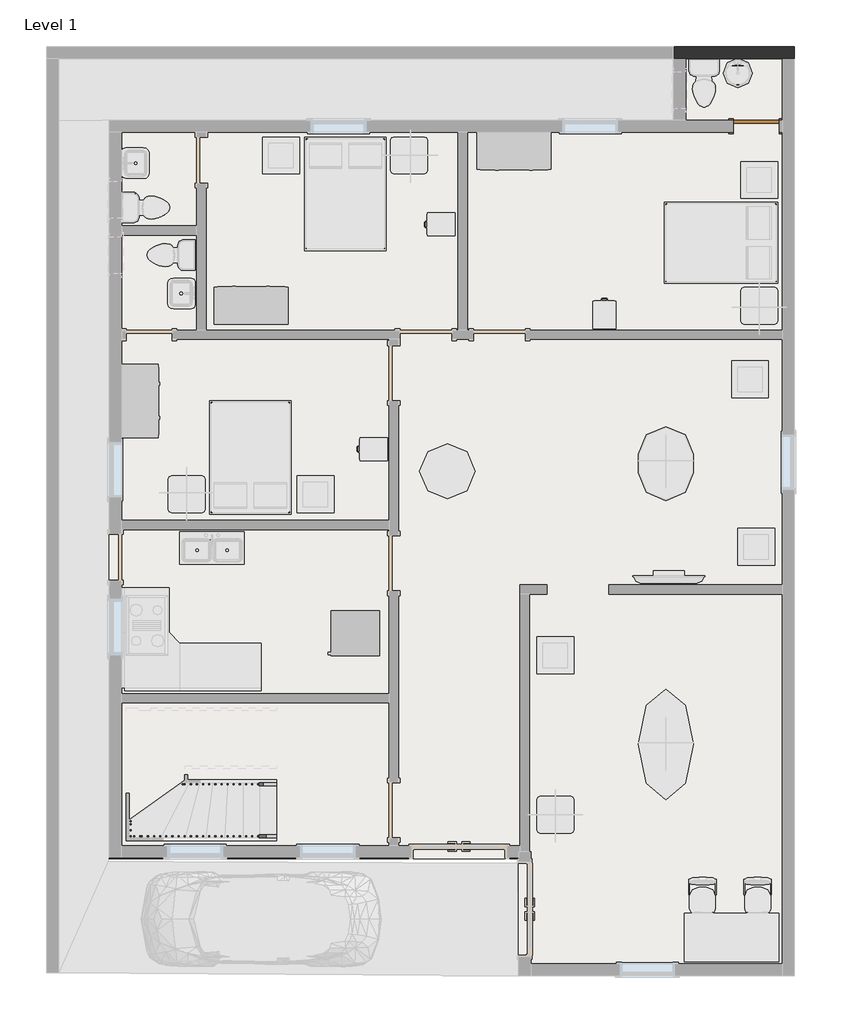
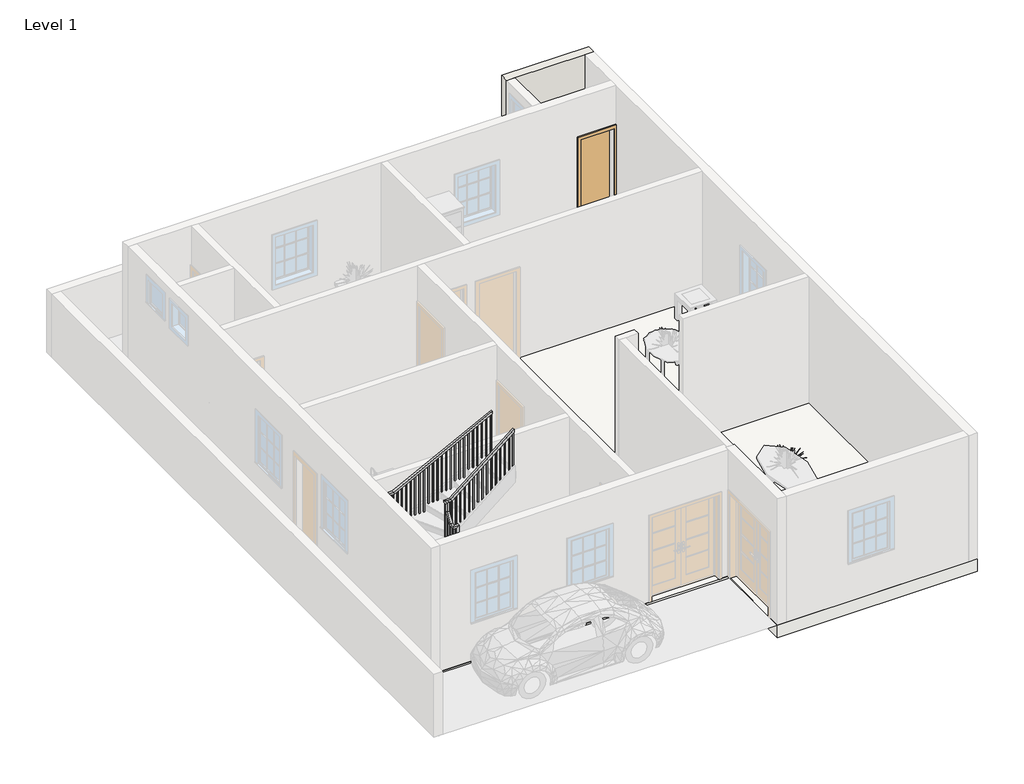
# One storey, part 2 of 3: 2 railings, 2 slabs, 1 door, 1 wall.
"""IFC4 building model written with IfcOpenShell, lengths in millimetres."""

from ifc_helpers import new_model, si_unit, frame, origin, place, context, project, spatial, polyline, outline, extrude, faceted_brep, transform, mapped, element, save
from components import door_fadea3f2

model = new_model("IFC4")

# Units and contexts
model_context = context("Model", 3, world=origin())
ifc_project = project(units=[si_unit("LENGTHUNIT", "METRE", prefix="MILLI")], contexts=[model_context])

# Site, building, storey
site = spatial("IfcSite", under=ifc_project)
building = spatial("IfcBuilding", under=site)
storey = spatial("IfcBuildingStorey", under=building, Name="Level 1", Elevation=0.0)

# Door
placement = place(None, origin())
door_shape = door_fadea3f2(model_context)
element("IfcDoor", 1, ObjectType="Single-Flush : 30\" x 80\"", at=placement, inside=storey, context=model_context, shape_type="MappedRepresentation", body=[
    mapped(door_shape, transform((2172.6442798, 14156.4245992, 0.0), x_axis=(1.0, 0.0, 0.0), y_axis=(0.0, 1.0, 0.0), z_axis=(0.0, 0.0, 1.0))),
])

# Railings
element("IfcRailing", 2, ObjectType="Handrail - Rectangular", at=placement, inside=storey, context=model_context, shape_type="SolidModel", body=[
    faceted_brep([(-5773.8240284, 3234.4245992, 1025.2529681), (-5773.8240284, 3234.4245992, 959.7067088), (-5773.8240284, 3285.2245992, 959.7067088), (-5773.8240284, 3285.2245992, 1025.2529681), (-7225.3557202, 3234.4245992, 2208.7848338), (-7276.1557202, 3234.4245992, 2184.659247), (-7276.1557202, 3285.2245992, 2184.659247), (-7225.3557202, 3285.2245992, 2208.7848338), (-7225.3557202, 3234.4245992, 2414.6281882), (-7276.1557202, 3234.4245992, 2363.8281882), (-7276.1557202, 3285.2245992, 2363.8281882), (-7225.3557202, 3285.2245992, 2414.6281882), (-7352.3557202, 3234.4245992, 2414.6281882), (-7352.3557202, 3234.4245992, 2363.8281882), (-7301.5557202, 3285.2245992, 2363.8281882), (-7301.5557202, 3285.2245992, 2414.6281882), (-7352.3557202, 3361.4245992, 2414.6281882), (-7352.3557202, 3390.5459331, 2363.8281882), (-7301.5557202, 3390.5459331, 2363.8281882), (-7301.5557202, 3361.4245992, 2414.6281882), (-7352.3557202, 3488.4245992, 2631.5051451), (-7352.3557202, 3539.2245992, 2617.7256424), (-7301.5557202, 3539.2245992, 2617.7256424), (-7301.5557202, 3488.4245992, 2631.5051451), (-7352.3557202, 3488.4245992, 2837.3484995), (-7352.3557202, 3539.2245992, 2786.5484995), (-7301.5557202, 3539.2245992, 2786.5484995), (-7301.5557202, 3488.4245992, 2837.3484995), (-7352.3557202, 3615.4245992, 2837.3484995), (-7352.3557202, 3615.4245992, 2786.5484995), (-7301.5557202, 3564.6245992, 2786.5484995), (-7301.5557202, 3564.6245992, 2837.3484995), (-7225.3557202, 3615.4245992, 2837.3484995), (-7207.2703071, 3615.4245992, 2786.5484995), (-7207.2703071, 3564.6245992, 2786.5484995), (-7225.3557202, 3564.6245992, 2837.3484995), (-5773.8240284, 3615.4245992, 4020.8803652), (-5773.8240284, 3564.6245992, 4020.8803652), (-5773.8240284, 3564.6245992, 3955.3341059), (-5773.8240284, 3615.4245992, 3955.3341059)], [[[0, 1, 2, 3]], [[1, 0, 4, 5]], [[2, 1, 5, 6]], [[3, 2, 6, 7]], [[0, 3, 7, 4]], [[5, 4, 8, 9]], [[6, 5, 9, 10]], [[7, 6, 10, 11]], [[4, 7, 11, 8]], [[9, 8, 12, 13]], [[10, 9, 13, 14]], [[11, 10, 14, 15]], [[8, 11, 15, 12]], [[13, 12, 16, 17]], [[14, 13, 17, 18]], [[15, 14, 18, 19]], [[12, 15, 19, 16]], [[17, 16, 20, 21]], [[18, 17, 21, 22]], [[19, 18, 22, 23]], [[16, 19, 23, 20]], [[21, 20, 24, 25]], [[22, 21, 25, 26]], [[23, 22, 26, 27]], [[20, 23, 27, 24]], [[25, 24, 28, 29]], [[26, 25, 29, 30]], [[27, 26, 30, 31]], [[24, 27, 31, 28]], [[29, 28, 32, 33]], [[30, 29, 33, 34]], [[31, 30, 34, 35]], [[28, 31, 35, 32]], [[36, 37, 38, 39]], [[33, 32, 36, 39]], [[34, 33, 39, 38]], [[35, 34, 38, 37]], [[32, 35, 37, 36]]]),
    extrude(outline(polyline([(3881.7558784, -5864.0633639), (3866.2231262, -5883.1133639), (2878.6666667, -5883.1133639), (2878.6666667, -5864.0633639), (3881.7558784, -5864.0633639)])), frame((0.0, 3580.4995992, 0.0), z_axis=(0.0, 1.0, 0.0), x_axis=(0.0, 0.0, 1.0)), (0.0, 0.0, 1.0), 19.05),
    extrude(outline(polyline([(3798.9145334, -5965.6633639), (3783.3817813, -5984.7133639), (2878.6666667, -5984.7133639), (2878.6666667, -5965.6633639), (3798.9145334, -5965.6633639)])), frame((0.0, 3580.4995992, 0.0), z_axis=(0.0, 1.0, 0.0), x_axis=(0.0, 0.0, 1.0)), (0.0, 0.0, 1.0), 19.05),
    extrude(outline(polyline([(3716.0731885, -6067.2633639), (3700.5404364, -6086.3133639), (2709.3333333, -6086.3133639), (2709.3333333, -6067.2633639), (3716.0731885, -6067.2633639)])), frame((0.0, 3580.4995992, 0.0), z_axis=(0.0, 1.0, 0.0), x_axis=(0.0, 0.0, 1.0)), (0.0, 0.0, 1.0), 19.05),
    extrude(outline(polyline([(3633.2318436, -6168.8633639), (3617.6990914, -6187.9133639), (2709.3333333, -6187.9133639), (2709.3333333, -6168.8633639), (3633.2318436, -6168.8633639)])), frame((0.0, 3580.4995992, 0.0), z_axis=(0.0, 1.0, 0.0), x_axis=(0.0, 0.0, 1.0)), (0.0, 0.0, 1.0), 19.05),
    extrude(outline(polyline([(3550.3904987, -6270.4633639), (3534.8577465, -6289.5133639), (2709.3333333, -6289.5133639), (2709.3333333, -6270.4633639), (3550.3904987, -6270.4633639)])), frame((0.0, 3580.4995992, 0.0), z_axis=(0.0, 1.0, 0.0), x_axis=(0.0, 0.0, 1.0)), (0.0, 0.0, 1.0), 19.05),
    extrude(outline(polyline([(3467.5491538, -6372.0633639), (3452.0164016, -6391.1133639), (2540.0, -6391.1133639), (2540.0, -6372.0633639), (3467.5491538, -6372.0633639)])), frame((0.0, 3580.4995992, 0.0), z_axis=(0.0, 1.0, 0.0), x_axis=(0.0, 0.0, 1.0)), (0.0, 0.0, 1.0), 19.05),
    extrude(outline(polyline([(3384.7078088, -6473.6633639), (3369.1750567, -6492.7133639), (2540.0, -6492.7133639), (2540.0, -6473.6633639), (3384.7078088, -6473.6633639)])), frame((0.0, 3580.4995992, 0.0), z_axis=(0.0, 1.0, 0.0), x_axis=(0.0, 0.0, 1.0)), (0.0, 0.0, 1.0), 19.05),
    extrude(outline(polyline([(3301.8664639, -6575.2633639), (3286.3337117, -6594.3133639), (2540.0, -6594.3133639), (2540.0, -6575.2633639), (3301.8664639, -6575.2633639)])), frame((0.0, 3580.4995992, 0.0), z_axis=(0.0, 1.0, 0.0), x_axis=(0.0, 0.0, 1.0)), (0.0, 0.0, 1.0), 19.05),
    extrude(outline(polyline([(3219.025119, -6676.8633639), (3203.4923668, -6695.9133639), (2370.6666667, -6695.9133639), (2370.6666667, -6676.8633639), (3219.025119, -6676.8633639)])), frame((0.0, 3580.4995992, 0.0), z_axis=(0.0, 1.0, 0.0), x_axis=(0.0, 0.0, 1.0)), (0.0, 0.0, 1.0), 19.05),
    extrude(outline(polyline([(3136.1837741, -6778.4633639), (3120.6510219, -6797.5133639), (2370.6666667, -6797.5133639), (2370.6666667, -6778.4633639), (3136.1837741, -6778.4633639)])), frame((0.0, 3580.4995992, 0.0), z_axis=(0.0, 1.0, 0.0), x_axis=(0.0, 0.0, 1.0)), (0.0, 0.0, 1.0), 19.05),
    extrude(outline(polyline([(3053.3424291, -6880.0633639), (3037.809677, -6899.1133639), (2201.3333333, -6899.1133639), (2201.3333333, -6880.0633639), (3053.3424291, -6880.0633639)])), frame((0.0, 3580.4995992, 0.0), z_axis=(0.0, 1.0, 0.0), x_axis=(0.0, 0.0, 1.0)), (0.0, 0.0, 1.0), 19.05),
    extrude(outline(polyline([(2970.5010842, -6981.6633639), (2954.9683321, -7000.7133639), (2201.3333333, -7000.7133639), (2201.3333333, -6981.6633639), (2970.5010842, -6981.6633639)])), frame((0.0, 3580.4995992, 0.0), z_axis=(0.0, 1.0, 0.0), x_axis=(0.0, 0.0, 1.0)), (0.0, 0.0, 1.0), 19.05),
    extrude(outline(polyline([(2887.6597393, -7083.2633639), (2872.1269871, -7102.3133639), (2032.0, -7102.3133639), (2032.0, -7083.2633639), (2887.6597393, -7083.2633639)])), frame((0.0, 3580.4995992, 0.0), z_axis=(0.0, 1.0, 0.0), x_axis=(0.0, 0.0, 1.0)), (0.0, 0.0, 1.0), 19.05),
    extrude(outline(polyline([(2804.8183944, -7184.8633639), (2789.2856422, -7203.9133639), (2032.0, -7203.9133639), (2032.0, -7184.8633639), (2804.8183944, -7184.8633639)])), frame((0.0, 3580.4995992, 0.0), z_axis=(0.0, 1.0, 0.0), x_axis=(0.0, 0.0, 1.0)), (0.0, 0.0, 1.0), 19.05),
    extrude(outline(polyline([(3468.285503, 2496.5834745), (3487.335503, 2529.115018), (3487.335503, 1524.0), (3468.285503, 1524.0), (3468.285503, 2496.5834745)])), frame((-7336.4807202, 0.0, 0.0), z_axis=(1.0, 0.0, 0.0), x_axis=(0.0, 1.0, 0.0)), (0.0, 0.0, 1.0), 19.05),
    extrude(outline(polyline([(3366.685503, 2323.0819089), (3385.735503, 2355.6134525), (3385.735503, 1524.0), (3366.685503, 1524.0), (3366.685503, 2323.0819089)])), frame((-7336.4807202, 0.0, 0.0), z_axis=(1.0, 0.0, 0.0), x_axis=(0.0, 1.0, 0.0)), (0.0, 0.0, 1.0), 19.05),
    extrude(outline(polyline([(2111.7191617, -7186.6990284), (2127.2519138, -7205.7490284), (1016.0, -7205.7490284), (1016.0, -7186.6990284), (2111.7191617, -7186.6990284)])), frame((0.0, 3250.2995992, 0.0), z_axis=(0.0, 1.0, 0.0), x_axis=(0.0, 0.0, 1.0)), (0.0, 0.0, 1.0), 19.05),
    extrude(outline(polyline([(2028.8778167, -7085.0990284), (2044.4105689, -7104.1490284), (1016.0, -7104.1490284), (1016.0, -7085.0990284), (2028.8778167, -7085.0990284)])), frame((0.0, 3250.2995992, 0.0), z_axis=(0.0, 1.0, 0.0), x_axis=(0.0, 0.0, 1.0)), (0.0, 0.0, 1.0), 19.05),
    extrude(outline(polyline([(1946.0364718, -6983.4990284), (1961.569224, -7002.5490284), (846.6666667, -7002.5490284), (846.6666667, -6983.4990284), (1946.0364718, -6983.4990284)])), frame((0.0, 3250.2995992, 0.0), z_axis=(0.0, 1.0, 0.0), x_axis=(0.0, 0.0, 1.0)), (0.0, 0.0, 1.0), 19.05),
    extrude(outline(polyline([(1863.1951269, -6881.8990284), (1878.7278791, -6900.9490284), (846.6666667, -6900.9490284), (846.6666667, -6881.8990284), (1863.1951269, -6881.8990284)])), frame((0.0, 3250.2995992, 0.0), z_axis=(0.0, 1.0, 0.0), x_axis=(0.0, 0.0, 1.0)), (0.0, 0.0, 1.0), 19.05),
    extrude(outline(polyline([(1780.353782, -6780.2990284), (1795.8865341, -6799.3490284), (677.3333333, -6799.3490284), (677.3333333, -6780.2990284), (1780.353782, -6780.2990284)])), frame((0.0, 3250.2995992, 0.0), z_axis=(0.0, 1.0, 0.0), x_axis=(0.0, 0.0, 1.0)), (0.0, 0.0, 1.0), 19.05),
    extrude(outline(polyline([(1697.5124371, -6678.6990284), (1713.0451892, -6697.7490284), (677.3333333, -6697.7490284), (677.3333333, -6678.6990284), (1697.5124371, -6678.6990284)])), frame((0.0, 3250.2995992, 0.0), z_axis=(0.0, 1.0, 0.0), x_axis=(0.0, 0.0, 1.0)), (0.0, 0.0, 1.0), 19.05),
    extrude(outline(polyline([(1614.6710921, -6577.0990284), (1630.2038443, -6596.1490284), (508.0, -6596.1490284), (508.0, -6577.0990284), (1614.6710921, -6577.0990284)])), frame((0.0, 3250.2995992, 0.0), z_axis=(0.0, 1.0, 0.0), x_axis=(0.0, 0.0, 1.0)), (0.0, 0.0, 1.0), 19.05),
    extrude(outline(polyline([(1531.8297472, -6475.4990284), (1547.3624994, -6494.5490284), (508.0, -6494.5490284), (508.0, -6475.4990284), (1531.8297472, -6475.4990284)])), frame((0.0, 3250.2995992, 0.0), z_axis=(0.0, 1.0, 0.0), x_axis=(0.0, 0.0, 1.0)), (0.0, 0.0, 1.0), 19.05),
    extrude(outline(polyline([(1448.9884023, -6373.8990284), (1464.5211545, -6392.9490284), (508.0, -6392.9490284), (508.0, -6373.8990284), (1448.9884023, -6373.8990284)])), frame((0.0, 3250.2995992, 0.0), z_axis=(0.0, 1.0, 0.0), x_axis=(0.0, 0.0, 1.0)), (0.0, 0.0, 1.0), 19.05),
    extrude(outline(polyline([(1366.1470574, -6272.2990284), (1381.6798095, -6291.3490284), (338.6666667, -6291.3490284), (338.6666667, -6272.2990284), (1366.1470574, -6272.2990284)])), frame((0.0, 3250.2995992, 0.0), z_axis=(0.0, 1.0, 0.0), x_axis=(0.0, 0.0, 1.0)), (0.0, 0.0, 1.0), 19.05),
    extrude(outline(polyline([(1283.3057124, -6170.6990284), (1298.8384646, -6189.7490284), (338.6666667, -6189.7490284), (338.6666667, -6170.6990284), (1283.3057124, -6170.6990284)])), frame((0.0, 3250.2995992, 0.0), z_axis=(0.0, 1.0, 0.0), x_axis=(0.0, 0.0, 1.0)), (0.0, 0.0, 1.0), 19.05),
    extrude(outline(polyline([(1200.4643675, -6069.0990284), (1215.9971197, -6088.1490284), (338.6666667, -6088.1490284), (338.6666667, -6069.0990284), (1200.4643675, -6069.0990284)])), frame((0.0, 3250.2995992, 0.0), z_axis=(0.0, 1.0, 0.0), x_axis=(0.0, 0.0, 1.0)), (0.0, 0.0, 1.0), 19.05),
    extrude(outline(polyline([(1117.6230226, -5967.4990284), (1133.1557748, -5986.5490284), (169.3333333, -5986.5490284), (169.3333333, -5967.4990284), (1117.6230226, -5967.4990284)])), frame((0.0, 3250.2995992, 0.0), z_axis=(0.0, 1.0, 0.0), x_axis=(0.0, 0.0, 1.0)), (0.0, 0.0, 1.0), 19.05),
    extrude(outline(polyline([(1034.7816777, -5865.8990284), (1050.3144298, -5884.9490284), (169.3333333, -5884.9490284), (169.3333333, -5865.8990284), (1034.7816777, -5865.8990284)])), frame((0.0, 3250.2995992, 0.0), z_axis=(0.0, 1.0, 0.0), x_axis=(0.0, 0.0, 1.0)), (0.0, 0.0, 1.0), 19.05),
    extrude(outline(polyline([(-7305.5133639, 3580.4995992), (-7305.5133639, 3599.5495992), (-7286.4633639, 3599.5495992), (-7286.4633639, 3580.4995992), (-7305.5133639, 3580.4995992)])), frame((0.0, 0.0, 1862.6666667), z_axis=(0.0, 0.0, 1.0), x_axis=(1.0, 0.0, 0.0)), (0.0, 0.0, 1.0), 923.8818329),
    extrude(outline(polyline([(-7317.4307202, 3580.4995992), (-7336.4807202, 3580.4995992), (-7336.4807202, 3599.5495992), (-7317.4307202, 3599.5495992), (-7317.4307202, 3580.4995992)])), frame((0.0, 0.0, 1862.6666667), z_axis=(0.0, 0.0, 1.0), x_axis=(1.0, 0.0, 0.0)), (0.0, 0.0, 1.0), 923.8818329),
    extrude(outline(polyline([(-7317.4307202, 3565.7136955), (-7336.4807202, 3565.7136955), (-7336.4807202, 3584.7636955), (-7317.4307202, 3584.7636955), (-7317.4307202, 3565.7136955)])), frame((0.0, 0.0, 1693.3333333), z_axis=(0.0, 0.0, 1.0), x_axis=(1.0, 0.0, 0.0)), (0.0, 0.0, 1.0), 1093.2151662),
    extrude(outline(polyline([(-7317.4307202, 3265.085503), (-7336.4807202, 3265.085503), (-7336.4807202, 3284.135503), (-7317.4307202, 3284.135503), (-7317.4307202, 3265.085503)])), frame((0.0, 0.0, 1354.6666667), z_axis=(0.0, 0.0, 1.0), x_axis=(1.0, 0.0, 0.0)), (0.0, 0.0, 1.0), 1009.1615215),
    extrude(outline(polyline([(-7317.4307202, 3269.3495992), (-7317.4307202, 3250.2995992), (-7336.4807202, 3250.2995992), (-7336.4807202, 3269.3495992), (-7317.4307202, 3269.3495992)])), frame((0.0, 0.0, 1185.3333333), z_axis=(0.0, 0.0, 1.0), x_axis=(1.0, 0.0, 0.0)), (0.0, 0.0, 1.0), 1178.4948549),
    extrude(outline(polyline([(-7286.4633639, 3269.3495992), (-7286.4633639, 3250.2995992), (-7305.5133639, 3250.2995992), (-7305.5133639, 3269.3495992), (-7286.4633639, 3269.3495992)])), frame((0.0, 0.0, 1185.3333333), z_axis=(0.0, 0.0, 1.0), x_axis=(1.0, 0.0, 0.0)), (0.0, 0.0, 1.0), 1178.4948549),
    extrude(outline(polyline([(3955.3341059, -5773.8240284), (3939.8013537, -5792.8740284), (2878.6666667, -5792.8740284), (2878.6666667, -5773.8240284), (3955.3341059, -5773.8240284)])), frame((0.0, 3580.4995992, 0.0), z_axis=(0.0, 1.0, 0.0), x_axis=(0.0, 0.0, 1.0)), (0.0, 0.0, 1.0), 19.05),
    extrude(outline(polyline([(959.7067088, -5773.8240284), (975.239461, -5792.8740284), (169.3333333, -5792.8740284), (169.3333333, -5773.8240284), (959.7067088, -5773.8240284)])), frame((0.0, 3250.2995992, 0.0), z_axis=(0.0, 1.0, 0.0), x_axis=(0.0, 0.0, 1.0)), (0.0, 0.0, 1.0), 19.05),
])
element("IfcRailing", 3, ObjectType="Handrail - Rectangular", at=placement, inside=storey, context=model_context, shape_type="SolidModel", body=[
    faceted_brep([(-5773.8240284, 2370.8245992, 1109.0771751), (-5773.8240284, 2370.8245992, 1051.9280057), (-5773.8240284, 2421.6245992, 1051.9280057), (-5773.8240284, 2421.6245992, 1109.0771751), (-8033.8058849, 2370.8245992, 2273.7644996), (-8046.1259362, 2370.8245992, 2222.9644996), (-8046.1259362, 2421.6245992, 2222.9644996), (-8033.8058849, 2421.6245992, 2273.7644996), (-8215.9557202, 2370.8245992, 2273.7644996), (-8215.9557202, 2370.8245992, 2222.9644996), (-8165.1557202, 2421.6245992, 2222.9644996), (-8165.1557202, 2421.6245992, 2273.7644996), (-8215.9557202, 2647.9785518, 2273.7644996), (-8215.9557202, 2655.929128, 2222.9644996), (-8165.1557202, 2655.929128, 2222.9644996), (-8165.1557202, 2647.9785518, 2273.7644996), (-8215.9557202, 4201.8706466, 2772.3688337), (-8215.9557202, 4209.8212227, 2721.5688337), (-8165.1557202, 4209.8212227, 2721.5688337), (-8165.1557202, 4201.8706466, 2772.3688337), (-8215.9557202, 4479.0245992, 2772.3688337), (-8215.9557202, 4479.0245992, 2721.5688337), (-8165.1557202, 4428.2245992, 2721.5688337), (-8165.1557202, 4428.2245992, 2772.3688337), (-8033.8058849, 4479.0245992, 2772.3688337), (-8021.4858336, 4479.0245992, 2721.5688337), (-8021.4858336, 4428.2245992, 2721.5688337), (-8033.8058849, 4428.2245992, 2772.3688337), (-5773.8240284, 4479.0245992, 3937.0561582), (-5773.8240284, 4428.2245992, 3937.0561582), (-5773.8240284, 4428.2245992, 3879.9069889), (-5773.8240284, 4479.0245992, 3879.9069889)], [[[0, 1, 2, 3]], [[1, 0, 4, 5]], [[2, 1, 5, 6]], [[3, 2, 6, 7]], [[0, 3, 7, 4]], [[5, 4, 8, 9]], [[6, 5, 9, 10]], [[7, 6, 10, 11]], [[4, 7, 11, 8]], [[9, 8, 12, 13]], [[10, 9, 13, 14]], [[11, 10, 14, 15]], [[8, 11, 15, 12]], [[13, 12, 16, 17]], [[14, 13, 17, 18]], [[15, 14, 18, 19]], [[12, 15, 19, 16]], [[17, 16, 20, 21]], [[18, 17, 21, 22]], [[19, 18, 22, 23]], [[16, 19, 23, 20]], [[21, 20, 24, 25]], [[22, 21, 25, 26]], [[23, 22, 26, 27]], [[20, 23, 27, 24]], [[28, 29, 30, 31]], [[25, 24, 28, 31]], [[26, 25, 31, 30]], [[27, 26, 30, 29]], [[24, 27, 29, 28]]]),
    extrude(outline(polyline([(3862.2268642, -5808.1308849), (2878.6666667, -5808.1308849), (2878.6666667, -5789.0808849), (3872.0443296, -5789.0808849), (3862.2268642, -5808.1308849)])), frame((0.0, 4444.0995992, 0.0), z_axis=(0.0, 1.0, 0.0), x_axis=(0.0, 0.0, 1.0)), (0.0, 0.0, 1.0), 19.05),
    extrude(outline(polyline([(3809.8670491, -5909.7308849), (2878.6666667, -5909.7308849), (2878.6666667, -5890.6808849), (3819.6845145, -5890.6808849), (3809.8670491, -5909.7308849)])), frame((0.0, 4444.0995992, 0.0), z_axis=(0.0, 1.0, 0.0), x_axis=(0.0, 0.0, 1.0)), (0.0, 0.0, 1.0), 19.05),
    extrude(outline(polyline([(3757.507234, -6011.3308849), (2878.6666667, -6011.3308849), (2878.6666667, -5992.2808849), (3767.3246993, -5992.2808849), (3757.507234, -6011.3308849)])), frame((0.0, 4444.0995992, 0.0), z_axis=(0.0, 1.0, 0.0), x_axis=(0.0, 0.0, 1.0)), (0.0, 0.0, 1.0), 19.05),
    extrude(outline(polyline([(3705.1474189, -6112.9308849), (2709.3333333, -6112.9308849), (2709.3333333, -6093.8808849), (3714.9648842, -6093.8808849), (3705.1474189, -6112.9308849)])), frame((0.0, 4444.0995992, 0.0), z_axis=(0.0, 1.0, 0.0), x_axis=(0.0, 0.0, 1.0)), (0.0, 0.0, 1.0), 19.05),
    extrude(outline(polyline([(3652.7876038, -6214.5308849), (2709.3333333, -6214.5308849), (2709.3333333, -6195.4808849), (3662.6050691, -6195.4808849), (3652.7876038, -6214.5308849)])), frame((0.0, 4444.0995992, 0.0), z_axis=(0.0, 1.0, 0.0), x_axis=(0.0, 0.0, 1.0)), (0.0, 0.0, 1.0), 19.05),
    extrude(outline(polyline([(3600.4277887, -6316.1308849), (2709.3333333, -6316.1308849), (2709.3333333, -6297.0808849), (3610.245254, -6297.0808849), (3600.4277887, -6316.1308849)])), frame((0.0, 4444.0995992, 0.0), z_axis=(0.0, 1.0, 0.0), x_axis=(0.0, 0.0, 1.0)), (0.0, 0.0, 1.0), 19.05),
    extrude(outline(polyline([(3548.0679735, -6417.7308849), (2540.0, -6417.7308849), (2540.0, -6398.6808849), (3557.8854389, -6398.6808849), (3548.0679735, -6417.7308849)])), frame((0.0, 4444.0995992, 0.0), z_axis=(0.0, 1.0, 0.0), x_axis=(0.0, 0.0, 1.0)), (0.0, 0.0, 1.0), 19.05),
    extrude(outline(polyline([(3495.7081584, -6519.3308849), (2540.0, -6519.3308849), (2540.0, -6500.2808849), (3505.5256238, -6500.2808849), (3495.7081584, -6519.3308849)])), frame((0.0, 4444.0995992, 0.0), z_axis=(0.0, 1.0, 0.0), x_axis=(0.0, 0.0, 1.0)), (0.0, 0.0, 1.0), 19.05),
    extrude(outline(polyline([(3443.3483433, -6620.9308849), (2540.0, -6620.9308849), (2540.0, -6601.8808849), (3453.1658086, -6601.8808849), (3443.3483433, -6620.9308849)])), frame((0.0, 4444.0995992, 0.0), z_axis=(0.0, 1.0, 0.0), x_axis=(0.0, 0.0, 1.0)), (0.0, 0.0, 1.0), 19.05),
    extrude(outline(polyline([(3390.9885282, -6722.5308849), (2370.6666667, -6722.5308849), (2370.6666667, -6703.4808849), (3400.8059935, -6703.4808849), (3390.9885282, -6722.5308849)])), frame((0.0, 4444.0995992, 0.0), z_axis=(0.0, 1.0, 0.0), x_axis=(0.0, 0.0, 1.0)), (0.0, 0.0, 1.0), 19.05),
    extrude(outline(polyline([(3338.6287131, -6824.1308849), (2370.6666667, -6824.1308849), (2370.6666667, -6805.0808849), (3348.4461784, -6805.0808849), (3338.6287131, -6824.1308849)])), frame((0.0, 4444.0995992, 0.0), z_axis=(0.0, 1.0, 0.0), x_axis=(0.0, 0.0, 1.0)), (0.0, 0.0, 1.0), 19.05),
    extrude(outline(polyline([(3286.268898, -6925.7308849), (2370.6666667, -6925.7308849), (2370.6666667, -6906.6808849), (3296.0863633, -6906.6808849), (3286.268898, -6925.7308849)])), frame((0.0, 4444.0995992, 0.0), z_axis=(0.0, 1.0, 0.0), x_axis=(0.0, 0.0, 1.0)), (0.0, 0.0, 1.0), 19.05),
    extrude(outline(polyline([(3233.9090828, -7027.3308849), (2201.3333333, -7027.3308849), (2201.3333333, -7008.2808849), (3243.7265482, -7008.2808849), (3233.9090828, -7027.3308849)])), frame((0.0, 4444.0995992, 0.0), z_axis=(0.0, 1.0, 0.0), x_axis=(0.0, 0.0, 1.0)), (0.0, 0.0, 1.0), 19.05),
    extrude(outline(polyline([(3181.5492677, -7128.9308849), (2201.3333333, -7128.9308849), (2201.3333333, -7109.8808849), (3191.3667331, -7109.8808849), (3181.5492677, -7128.9308849)])), frame((0.0, 4444.0995992, 0.0), z_axis=(0.0, 1.0, 0.0), x_axis=(0.0, 0.0, 1.0)), (0.0, 0.0, 1.0), 19.05),
    extrude(outline(polyline([(3129.1894526, -7230.5308849), (2201.3333333, -7230.5308849), (2201.3333333, -7211.4808849), (3139.0069179, -7211.4808849), (3129.1894526, -7230.5308849)])), frame((0.0, 4444.0995992, 0.0), z_axis=(0.0, 1.0, 0.0), x_axis=(0.0, 0.0, 1.0)), (0.0, 0.0, 1.0), 19.05),
    extrude(outline(polyline([(3076.8296375, -7332.1308849), (2032.0, -7332.1308849), (2032.0, -7313.0808849), (3086.6471028, -7313.0808849), (3076.8296375, -7332.1308849)])), frame((0.0, 4444.0995992, 0.0), z_axis=(0.0, 1.0, 0.0), x_axis=(0.0, 0.0, 1.0)), (0.0, 0.0, 1.0), 19.05),
    extrude(outline(polyline([(3024.4698224, -7433.7308849), (2032.0, -7433.7308849), (2032.0, -7414.6808849), (3034.2872877, -7414.6808849), (3024.4698224, -7433.7308849)])), frame((0.0, 4444.0995992, 0.0), z_axis=(0.0, 1.0, 0.0), x_axis=(0.0, 0.0, 1.0)), (0.0, 0.0, 1.0), 19.05),
    extrude(outline(polyline([(2972.1100073, -7535.3308849), (2032.0, -7535.3308849), (2032.0, -7516.2808849), (2981.9274726, -7516.2808849), (2972.1100073, -7535.3308849)])), frame((0.0, 4444.0995992, 0.0), z_axis=(0.0, 1.0, 0.0), x_axis=(0.0, 0.0, 1.0)), (0.0, 0.0, 1.0), 19.05),
    extrude(outline(polyline([(2919.7501921, -7636.9308849), (2032.0, -7636.9308849), (2032.0, -7617.8808849), (2929.5676575, -7617.8808849), (2919.7501921, -7636.9308849)])), frame((0.0, 4444.0995992, 0.0), z_axis=(0.0, 1.0, 0.0), x_axis=(0.0, 0.0, 1.0)), (0.0, 0.0, 1.0), 19.05),
    extrude(outline(polyline([(2867.390377, -7738.5308849), (1862.6666667, -7738.5308849), (1862.6666667, -7719.4808849), (2877.2078424, -7719.4808849), (2867.390377, -7738.5308849)])), frame((0.0, 4444.0995992, 0.0), z_axis=(0.0, 1.0, 0.0), x_axis=(0.0, 0.0, 1.0)), (0.0, 0.0, 1.0), 19.05),
    extrude(outline(polyline([(2815.0305619, -7840.1308849), (1862.6666667, -7840.1308849), (1862.6666667, -7821.0808849), (2824.8480272, -7821.0808849), (2815.0305619, -7840.1308849)])), frame((0.0, 4444.0995992, 0.0), z_axis=(0.0, 1.0, 0.0), x_axis=(0.0, 0.0, 1.0)), (0.0, 0.0, 1.0), 19.05),
    extrude(outline(polyline([(2762.6707468, -7941.7308849), (1862.6666667, -7941.7308849), (1862.6666667, -7922.6808849), (2772.4882121, -7922.6808849), (2762.6707468, -7941.7308849)])), frame((0.0, 4444.0995992, 0.0), z_axis=(0.0, 1.0, 0.0), x_axis=(0.0, 0.0, 1.0)), (0.0, 0.0, 1.0), 19.05),
    extrude(outline(polyline([(-8098.4807202, 4463.1495992), (-8079.4307202, 4463.1495992), (-8079.4307202, 4444.0995992), (-8098.4807202, 4444.0995992), (-8098.4807202, 4463.1495992)])), frame((0.0, 0.0, 1862.6666667), z_axis=(0.0, 0.0, 1.0), x_axis=(1.0, 0.0, 0.0)), (0.0, 0.0, 1.0), 858.902167),
    extrude(outline(polyline([(-8200.0807202, 4395.5456466), (-8200.0807202, 4414.5956466), (-8181.0307202, 4414.5956466), (-8181.0307202, 4395.5456466), (-8200.0807202, 4395.5456466)])), frame((0.0, 0.0, 1862.6666667), z_axis=(0.0, 0.0, 1.0), x_axis=(1.0, 0.0, 0.0)), (0.0, 0.0, 1.0), 858.902167),
    extrude(outline(polyline([(-8200.0807202, 4293.9456466), (-8200.0807202, 4312.9956466), (-8181.0307202, 4312.9956466), (-8181.0307202, 4293.9456466), (-8200.0807202, 4293.9456466)])), frame((0.0, 0.0, 1862.6666667), z_axis=(0.0, 0.0, 1.0), x_axis=(1.0, 0.0, 0.0)), (0.0, 0.0, 1.0), 858.902167),
    extrude(outline(polyline([(4181.5035518, 2712.4824155), (4181.5035518, 1693.3333333), (4162.4535518, 1693.3333333), (4162.4535518, 2706.3697564), (4181.5035518, 2712.4824155)])), frame((-8200.0807202, 0.0, 0.0), z_axis=(1.0, 0.0, 0.0), x_axis=(0.0, 1.0, 0.0)), (0.0, 0.0, 1.0), 19.05),
    extrude(outline(polyline([(4079.9035518, 2679.8815673), (4079.9035518, 1693.3333333), (4060.8535518, 1693.3333333), (4060.8535518, 2673.7689082), (4079.9035518, 2679.8815673)])), frame((-8200.0807202, 0.0, 0.0), z_axis=(1.0, 0.0, 0.0), x_axis=(0.0, 1.0, 0.0)), (0.0, 0.0, 1.0), 19.05),
    extrude(outline(polyline([(3978.3035518, 2647.280719), (3978.3035518, 1693.3333333), (3959.2535518, 1693.3333333), (3959.2535518, 2641.16806), (3978.3035518, 2647.280719)])), frame((-8200.0807202, 0.0, 0.0), z_axis=(1.0, 0.0, 0.0), x_axis=(0.0, 1.0, 0.0)), (0.0, 0.0, 1.0), 19.05),
    extrude(outline(polyline([(3876.7035518, 2614.6798708), (3876.7035518, 1693.3333333), (3857.6535518, 1693.3333333), (3857.6535518, 2608.5672118), (3876.7035518, 2614.6798708)])), frame((-8200.0807202, 0.0, 0.0), z_axis=(1.0, 0.0, 0.0), x_axis=(0.0, 1.0, 0.0)), (0.0, 0.0, 1.0), 19.05),
    extrude(outline(polyline([(3775.1035518, 2582.0790226), (3775.1035518, 1693.3333333), (3756.0535518, 1693.3333333), (3756.0535518, 2575.9663635), (3775.1035518, 2582.0790226)])), frame((-8200.0807202, 0.0, 0.0), z_axis=(1.0, 0.0, 0.0), x_axis=(0.0, 1.0, 0.0)), (0.0, 0.0, 1.0), 19.05),
    extrude(outline(polyline([(3673.5035518, 2549.4781744), (3673.5035518, 1693.3333333), (3654.4535518, 1693.3333333), (3654.4535518, 2543.3655153), (3673.5035518, 2549.4781744)])), frame((-8200.0807202, 0.0, 0.0), z_axis=(1.0, 0.0, 0.0), x_axis=(0.0, 1.0, 0.0)), (0.0, 0.0, 1.0), 19.05),
    extrude(outline(polyline([(3571.9035518, 2516.8773261), (3571.9035518, 1524.0), (3552.8535518, 1524.0), (3552.8535518, 2510.7646671), (3571.9035518, 2516.8773261)])), frame((-8200.0807202, 0.0, 0.0), z_axis=(1.0, 0.0, 0.0), x_axis=(0.0, 1.0, 0.0)), (0.0, 0.0, 1.0), 19.05),
    extrude(outline(polyline([(3470.3035518, 2484.2764779), (3470.3035518, 1524.0), (3451.2535518, 1524.0), (3451.2535518, 2478.1638189), (3470.3035518, 2484.2764779)])), frame((-8200.0807202, 0.0, 0.0), z_axis=(1.0, 0.0, 0.0), x_axis=(0.0, 1.0, 0.0)), (0.0, 0.0, 1.0), 19.05),
    extrude(outline(polyline([(3368.7035518, 2451.6756297), (3368.7035518, 1524.0), (3349.6535518, 1524.0), (3349.6535518, 2445.5629706), (3368.7035518, 2451.6756297)])), frame((-8200.0807202, 0.0, 0.0), z_axis=(1.0, 0.0, 0.0), x_axis=(0.0, 1.0, 0.0)), (0.0, 0.0, 1.0), 19.05),
    extrude(outline(polyline([(3267.1035518, 2419.0747814), (3267.1035518, 1524.0), (3248.0535518, 1524.0), (3248.0535518, 2412.9621224), (3267.1035518, 2419.0747814)])), frame((-8200.0807202, 0.0, 0.0), z_axis=(1.0, 0.0, 0.0), x_axis=(0.0, 1.0, 0.0)), (0.0, 0.0, 1.0), 19.05),
    extrude(outline(polyline([(3165.5035518, 2386.4739332), (3165.5035518, 1354.6666667), (3146.4535518, 1354.6666667), (3146.4535518, 2380.3612742), (3165.5035518, 2386.4739332)])), frame((-8200.0807202, 0.0, 0.0), z_axis=(1.0, 0.0, 0.0), x_axis=(0.0, 1.0, 0.0)), (0.0, 0.0, 1.0), 19.05),
    extrude(outline(polyline([(3063.9035518, 2353.873085), (3063.9035518, 1354.6666667), (3044.8535518, 1354.6666667), (3044.8535518, 2347.7604259), (3063.9035518, 2353.873085)])), frame((-8200.0807202, 0.0, 0.0), z_axis=(1.0, 0.0, 0.0), x_axis=(0.0, 1.0, 0.0)), (0.0, 0.0, 1.0), 19.05),
    extrude(outline(polyline([(2962.3035518, 2321.2722368), (2962.3035518, 1354.6666667), (2943.2535518, 1354.6666667), (2943.2535518, 2315.1595777), (2962.3035518, 2321.2722368)])), frame((-8200.0807202, 0.0, 0.0), z_axis=(1.0, 0.0, 0.0), x_axis=(0.0, 1.0, 0.0)), (0.0, 0.0, 1.0), 19.05),
    extrude(outline(polyline([(2860.7035518, 2288.6713885), (2860.7035518, 1354.6666667), (2841.6535518, 1354.6666667), (2841.6535518, 2282.5587295), (2860.7035518, 2288.6713885)])), frame((-8200.0807202, 0.0, 0.0), z_axis=(1.0, 0.0, 0.0), x_axis=(0.0, 1.0, 0.0)), (0.0, 0.0, 1.0), 19.05),
    extrude(outline(polyline([(2759.1035518, 2256.0705403), (2759.1035518, 1354.6666667), (2740.0535518, 1354.6666667), (2740.0535518, 2249.9578813), (2759.1035518, 2256.0705403)])), frame((-8200.0807202, 0.0, 0.0), z_axis=(1.0, 0.0, 0.0), x_axis=(0.0, 1.0, 0.0)), (0.0, 0.0, 1.0), 19.05),
    extrude(outline(polyline([(-8200.0807202, 2589.8995992), (-8200.0807202, 2608.9495992), (-8181.0307202, 2608.9495992), (-8181.0307202, 2589.8995992), (-8200.0807202, 2589.8995992)])), frame((0.0, 0.0, 1185.3333333), z_axis=(0.0, 0.0, 1.0), x_axis=(1.0, 0.0, 0.0)), (0.0, 0.0, 1.0), 1037.6311663),
    extrude(outline(polyline([(-8200.0807202, 2488.2995992), (-8200.0807202, 2507.3495992), (-8181.0307202, 2507.3495992), (-8181.0307202, 2488.2995992), (-8200.0807202, 2488.2995992)])), frame((0.0, 0.0, 1185.3333333), z_axis=(0.0, 0.0, 1.0), x_axis=(1.0, 0.0, 0.0)), (0.0, 0.0, 1.0), 1037.6311663),
    extrude(outline(polyline([(-8125.8808849, 2386.6995992), (-8144.9308849, 2386.6995992), (-8144.9308849, 2405.7495992), (-8125.8808849, 2405.7495992), (-8125.8808849, 2386.6995992)])), frame((0.0, 0.0, 1185.3333333), z_axis=(0.0, 0.0, 1.0), x_axis=(1.0, 0.0, 0.0)), (0.0, 0.0, 1.0), 1037.6311663),
    extrude(outline(polyline([(2208.752671, -8018.5490284), (1185.3333333, -8018.5490284), (1185.3333333, -7999.4990284), (2198.9352056, -7999.4990284), (2208.752671, -8018.5490284)])), frame((0.0, 2386.6995992, 0.0), z_axis=(0.0, 1.0, 0.0), x_axis=(0.0, 0.0, 1.0)), (0.0, 0.0, 1.0), 19.05),
    extrude(outline(polyline([(2156.3928558, -7916.9490284), (1185.3333333, -7916.9490284), (1185.3333333, -7897.8990284), (2146.5753905, -7897.8990284), (2156.3928558, -7916.9490284)])), frame((0.0, 2386.6995992, 0.0), z_axis=(0.0, 1.0, 0.0), x_axis=(0.0, 0.0, 1.0)), (0.0, 0.0, 1.0), 19.05),
    extrude(outline(polyline([(2104.0330407, -7815.3490284), (1185.3333333, -7815.3490284), (1185.3333333, -7796.2990284), (2094.2155754, -7796.2990284), (2104.0330407, -7815.3490284)])), frame((0.0, 2386.6995992, 0.0), z_axis=(0.0, 1.0, 0.0), x_axis=(0.0, 0.0, 1.0)), (0.0, 0.0, 1.0), 19.05),
    extrude(outline(polyline([(2051.6732256, -7713.7490284), (1185.3333333, -7713.7490284), (1185.3333333, -7694.6990284), (2041.8557603, -7694.6990284), (2051.6732256, -7713.7490284)])), frame((0.0, 2386.6995992, 0.0), z_axis=(0.0, 1.0, 0.0), x_axis=(0.0, 0.0, 1.0)), (0.0, 0.0, 1.0), 19.05),
    extrude(outline(polyline([(1999.3134105, -7612.1490284), (1016.0, -7612.1490284), (1016.0, -7593.0990284), (1989.4959452, -7593.0990284), (1999.3134105, -7612.1490284)])), frame((0.0, 2386.6995992, 0.0), z_axis=(0.0, 1.0, 0.0), x_axis=(0.0, 0.0, 1.0)), (0.0, 0.0, 1.0), 19.05),
    extrude(outline(polyline([(1946.9535954, -7510.5490284), (1016.0, -7510.5490284), (1016.0, -7491.4990284), (1937.13613, -7491.4990284), (1946.9535954, -7510.5490284)])), frame((0.0, 2386.6995992, 0.0), z_axis=(0.0, 1.0, 0.0), x_axis=(0.0, 0.0, 1.0)), (0.0, 0.0, 1.0), 19.05),
    extrude(outline(polyline([(1894.5937803, -7408.9490284), (1016.0, -7408.9490284), (1016.0, -7389.8990284), (1884.7763149, -7389.8990284), (1894.5937803, -7408.9490284)])), frame((0.0, 2386.6995992, 0.0), z_axis=(0.0, 1.0, 0.0), x_axis=(0.0, 0.0, 1.0)), (0.0, 0.0, 1.0), 19.05),
    extrude(outline(polyline([(1842.2339651, -7307.3490284), (1016.0, -7307.3490284), (1016.0, -7288.2990284), (1832.4164998, -7288.2990284), (1842.2339651, -7307.3490284)])), frame((0.0, 2386.6995992, 0.0), z_axis=(0.0, 1.0, 0.0), x_axis=(0.0, 0.0, 1.0)), (0.0, 0.0, 1.0), 19.05),
    extrude(outline(polyline([(1789.87415, -7205.7490284), (846.6666667, -7205.7490284), (846.6666667, -7186.6990284), (1780.0566847, -7186.6990284), (1789.87415, -7205.7490284)])), frame((0.0, 2386.6995992, 0.0), z_axis=(0.0, 1.0, 0.0), x_axis=(0.0, 0.0, 1.0)), (0.0, 0.0, 1.0), 19.05),
    extrude(outline(polyline([(1737.5143349, -7104.1490284), (846.6666667, -7104.1490284), (846.6666667, -7085.0990284), (1727.6968696, -7085.0990284), (1737.5143349, -7104.1490284)])), frame((0.0, 2386.6995992, 0.0), z_axis=(0.0, 1.0, 0.0), x_axis=(0.0, 0.0, 1.0)), (0.0, 0.0, 1.0), 19.05),
    extrude(outline(polyline([(1685.1545198, -7002.5490284), (846.6666667, -7002.5490284), (846.6666667, -6983.4990284), (1675.3370545, -6983.4990284), (1685.1545198, -7002.5490284)])), frame((0.0, 2386.6995992, 0.0), z_axis=(0.0, 1.0, 0.0), x_axis=(0.0, 0.0, 1.0)), (0.0, 0.0, 1.0), 19.05),
    extrude(outline(polyline([(1632.7947047, -6900.9490284), (677.3333333, -6900.9490284), (677.3333333, -6881.8990284), (1622.9772393, -6881.8990284), (1632.7947047, -6900.9490284)])), frame((0.0, 2386.6995992, 0.0), z_axis=(0.0, 1.0, 0.0), x_axis=(0.0, 0.0, 1.0)), (0.0, 0.0, 1.0), 19.05),
    extrude(outline(polyline([(1580.4348896, -6799.3490284), (677.3333333, -6799.3490284), (677.3333333, -6780.2990284), (1570.6174242, -6780.2990284), (1580.4348896, -6799.3490284)])), frame((0.0, 2386.6995992, 0.0), z_axis=(0.0, 1.0, 0.0), x_axis=(0.0, 0.0, 1.0)), (0.0, 0.0, 1.0), 19.05),
    extrude(outline(polyline([(1528.0750744, -6697.7490284), (677.3333333, -6697.7490284), (677.3333333, -6678.6990284), (1518.2576091, -6678.6990284), (1528.0750744, -6697.7490284)])), frame((0.0, 2386.6995992, 0.0), z_axis=(0.0, 1.0, 0.0), x_axis=(0.0, 0.0, 1.0)), (0.0, 0.0, 1.0), 19.05),
    extrude(outline(polyline([(1475.7152593, -6596.1490284), (508.0, -6596.1490284), (508.0, -6577.0990284), (1465.897794, -6577.0990284), (1475.7152593, -6596.1490284)])), frame((0.0, 2386.6995992, 0.0), z_axis=(0.0, 1.0, 0.0), x_axis=(0.0, 0.0, 1.0)), (0.0, 0.0, 1.0), 19.05),
    extrude(outline(polyline([(1423.3554442, -6494.5490284), (508.0, -6494.5490284), (508.0, -6475.4990284), (1413.5379789, -6475.4990284), (1423.3554442, -6494.5490284)])), frame((0.0, 2386.6995992, 0.0), z_axis=(0.0, 1.0, 0.0), x_axis=(0.0, 0.0, 1.0)), (0.0, 0.0, 1.0), 19.05),
    extrude(outline(polyline([(1370.9956291, -6392.9490284), (508.0, -6392.9490284), (508.0, -6373.8990284), (1361.1781638, -6373.8990284), (1370.9956291, -6392.9490284)])), frame((0.0, 2386.6995992, 0.0), z_axis=(0.0, 1.0, 0.0), x_axis=(0.0, 0.0, 1.0)), (0.0, 0.0, 1.0), 19.05),
    extrude(outline(polyline([(1318.635814, -6291.3490284), (338.6666667, -6291.3490284), (338.6666667, -6272.2990284), (1308.8183486, -6272.2990284), (1318.635814, -6291.3490284)])), frame((0.0, 2386.6995992, 0.0), z_axis=(0.0, 1.0, 0.0), x_axis=(0.0, 0.0, 1.0)), (0.0, 0.0, 1.0), 19.05),
    extrude(outline(polyline([(1266.2759989, -6189.7490284), (338.6666667, -6189.7490284), (338.6666667, -6170.6990284), (1256.4585335, -6170.6990284), (1266.2759989, -6189.7490284)])), frame((0.0, 2386.6995992, 0.0), z_axis=(0.0, 1.0, 0.0), x_axis=(0.0, 0.0, 1.0)), (0.0, 0.0, 1.0), 19.05),
    extrude(outline(polyline([(1213.9161837, -6088.1490284), (338.6666667, -6088.1490284), (338.6666667, -6069.0990284), (1204.0987184, -6069.0990284), (1213.9161837, -6088.1490284)])), frame((0.0, 2386.6995992, 0.0), z_axis=(0.0, 1.0, 0.0), x_axis=(0.0, 0.0, 1.0)), (0.0, 0.0, 1.0), 19.05),
    extrude(outline(polyline([(1161.5563686, -5986.5490284), (169.3333333, -5986.5490284), (169.3333333, -5967.4990284), (1151.7389033, -5967.4990284), (1161.5563686, -5986.5490284)])), frame((0.0, 2386.6995992, 0.0), z_axis=(0.0, 1.0, 0.0), x_axis=(0.0, 0.0, 1.0)), (0.0, 0.0, 1.0), 19.05),
    extrude(outline(polyline([(1109.1965535, -5884.9490284), (169.3333333, -5884.9490284), (169.3333333, -5865.8990284), (1099.3790882, -5865.8990284), (1109.1965535, -5884.9490284)])), frame((0.0, 2386.6995992, 0.0), z_axis=(0.0, 1.0, 0.0), x_axis=(0.0, 0.0, 1.0)), (0.0, 0.0, 1.0), 19.05),
    extrude(outline(polyline([(-8043.3308849, 4463.1495992), (-8024.2808849, 4463.1495992), (-8024.2808849, 4444.0995992), (-8043.3308849, 4444.0995992), (-8043.3308849, 4463.1495992)])), frame((0.0, 0.0, 1862.6666667), z_axis=(0.0, 0.0, 1.0), x_axis=(1.0, 0.0, 0.0)), (0.0, 0.0, 1.0), 858.902167),
    extrude(outline(polyline([(-8200.0807202, 4444.0995992), (-8200.0807202, 4463.1495992), (-8181.0307202, 4463.1495992), (-8181.0307202, 4444.0995992), (-8200.0807202, 4444.0995992)])), frame((0.0, 0.0, 1862.6666667), z_axis=(0.0, 0.0, 1.0), x_axis=(1.0, 0.0, 0.0)), (0.0, 0.0, 1.0), 858.902167),
    extrude(outline(polyline([(4211.3956466, 2722.0740262), (4211.3956466, 1862.6666667), (4192.3456466, 1862.6666667), (4192.3456466, 2715.9613671), (4211.3956466, 2722.0740262)])), frame((-8200.0807202, 0.0, 0.0), z_axis=(1.0, 0.0, 0.0), x_axis=(0.0, 1.0, 0.0)), (0.0, 0.0, 1.0), 19.05),
    extrude(outline(polyline([(-8200.0807202, 2638.4535518), (-8200.0807202, 2657.5035518), (-8181.0307202, 2657.5035518), (-8181.0307202, 2638.4535518), (-8200.0807202, 2638.4535518)])), frame((0.0, 0.0, 1185.3333333), z_axis=(0.0, 0.0, 1.0), x_axis=(1.0, 0.0, 0.0)), (0.0, 0.0, 1.0), 1037.6311663),
    extrude(outline(polyline([(-8181.0307202, 2386.6995992), (-8200.0807202, 2386.6995992), (-8200.0807202, 2405.7495992), (-8181.0307202, 2405.7495992), (-8181.0307202, 2386.6995992)])), frame((0.0, 0.0, 1185.3333333), z_axis=(0.0, 0.0, 1.0), x_axis=(1.0, 0.0, 0.0)), (0.0, 0.0, 1.0), 1037.6311663),
    extrude(outline(polyline([(2221.5240629, -8043.3308849), (1185.3333333, -8043.3308849), (1185.3333333, -8024.2808849), (2211.7065976, -8024.2808849), (2221.5240629, -8043.3308849)])), frame((0.0, 2386.6995992, 0.0), z_axis=(0.0, 1.0, 0.0), x_axis=(0.0, 0.0, 1.0)), (0.0, 0.0, 1.0), 19.05),
    extrude(outline(polyline([(3870.0895235, -5792.8740284), (2878.6666667, -5792.8740284), (2878.6666667, -5773.8240284), (3879.9069889, -5773.8240284), (3870.0895235, -5792.8740284)])), frame((0.0, 4444.0995992, 0.0), z_axis=(0.0, 1.0, 0.0), x_axis=(0.0, 0.0, 1.0)), (0.0, 0.0, 1.0), 19.05),
    extrude(outline(polyline([(1061.7454711, -5792.8740284), (169.3333333, -5792.8740284), (169.3333333, -5773.8240284), (1051.9280057, -5773.8240284), (1061.7454711, -5792.8740284)])), frame((0.0, 2386.6995992, 0.0), z_axis=(0.0, 1.0, 0.0), x_axis=(0.0, 0.0, 1.0)), (0.0, 0.0, 1.0), 19.05),
])

# Slabs
element("IfcSlab", 4, ObjectType="Generic - 12\"", at=placement, inside=storey, context=model_context, shape_type="SweptSolid", body=[
    extrude(outline(polyline([(2807.6442798, 14258.0245992), (2807.6442798, 84.8245992), (-1764.3557202, 84.8245992), (-1764.3557202, 2021.5745992), (-8546.1557202, 2021.5745992), (-8546.1557202, 14258.0245992), (2807.6442798, 14258.0245992)])), frame((0.0, 0.0, -304.8), z_axis=(0.0, 0.0, 1.0), x_axis=(1.0, 0.0, 0.0)), (0.0, 0.0, 1.0), 304.8),
])
element("IfcSlab", 5, ObjectType="Generic - 12\"", at=placement, inside=storey, context=model_context, shape_type="SweptSolid", body=[
    extrude(outline(polyline([(2807.6442798, 15477.2245992), (2807.6442798, 14258.0245992), (813.7442798, 14258.0245992), (813.7442798, 15477.2245992), (2807.6442798, 15477.2245992)])), frame((0.0, 0.0, -304.8), z_axis=(0.0, 0.0, 1.0), x_axis=(1.0, 0.0, 0.0)), (0.0, 0.0, 1.0), 304.8),
])

# Wall
element("IfcWall", 6, ObjectType="Generic - 8\"", at=placement, inside=storey, context=model_context, shape_type="Brep", body=[
    faceted_brep([(813.7442798, 15274.0245992, 0.0), (1004.2442798, 15274.0245992, 0.0), (2604.4442798, 15274.0245992, 0.0), (2807.6442798, 15274.0245992, 0.0), (2807.6442798, 15274.0245992, 3048.0), (2604.4442798, 15274.0245992, 3048.0), (1004.2442798, 15274.0245992, 3048.0), (813.7442798, 15274.0245992, 3048.0), (813.7442798, 15477.2245992, 0.0), (813.7442798, 15477.2245992, 3048.0), (2807.6442798, 15477.2245992, 3048.0), (2807.6442798, 15477.2245992, 0.0)], [[[0, 1, 2, 3, 4, 5, 6, 7]], [[8, 9, 10, 11]], [[3, 2, 1, 0, 8, 11]], [[0, 7, 9, 8]], [[4, 3, 11, 10]], [[7, 6, 5, 4, 10, 9]]]),
])

save(model, "model.ifc")

# Revit data of these elements
# Type "Single-Flush : 30\" x 80\""
#   Type Mark = "5"
#   Construction Type Id = "MDOOR"
#   Assembly Code = "C1020"
#   Analytic Construction = "Metal"
#   Thickness = 0' - 2"
#   Heat Transfer Coefficient (U) = 0.651978 BTU/(h·ft²·°F)
#   Height = 6' - 8"
#   Trim Projection Ext = 0' - 1"
#   Trim Projection Int = 0' - 1"
#   Trim Width = 0' - 3"
#   Width = 2' - 6"
#   Define Thermal Properties by = 1
#   Door Material = Door - Panel
#   Frame Material = Door - Frame
#   Visual Light Transmittance = 0
#   Solar Heat Gain Coefficient = 0
#   Function = (empty or 0)
#   Wall Closure = (empty or 0)
# Type "Handrail - Rectangular"
#   Assembly Code = "C2010400"
#   built-in parameter 1008612 = 0.0416667 (stored number, unit not read)
#   built-in parameter 1008611 = 0.0416667 (stored number, unit not read)
#   built-in parameter 1008609 = 0.333333 (stored number, unit not read)
#   built-in parameter 1008604 = 0.166667 (stored number, unit not read)
#   built-in parameter 1008603 = 0.166667 (stored number, unit not read)
#   Railing Height = 3' - 0"
#   built-in parameter 1008630 = 2
#   built-in parameter 1008610 = 2
#   built-in parameter 1008618 = Baluster - Square : 3/4"
# Type "Generic - 12\""
#   Assembly Code = "B1010"
#   Function = 0
#   Layers, outside or top first: 1' - 0" no material (function 1)
# Type "Generic - 8\""
#   Assembly Code = "B2010"
#   Layers, outside or top first: 0' - 8" "Brick, Common" (function 1)
# Element 1 (IfcDoor, "Single-Flush : 30\" x 80\"")
#   Phase Created = New Construction
#   Materials on its faces: "Door - Frame", "Door - Panel"
# Elements 2, 3 (IfcRailing, "Handrail - Rectangular")
#   Phase Created = New Construction
# Elements 4, 5 (IfcSlab, "Generic - 12\"")
#   Height Offset From Level = 0' - 0"
#   Phase Created = New Construction
#   Materials on its faces: "Default Floor"
# Element 6 (IfcWall, "Generic - 8\"")
#   Top Offset = 0' - 0"
#   Base Offset = 0' - 0"
#   Unconnected Height = 10' - 0"
#   wall height = 10' - 0"
#   Phase Created = New Construction
#   Base Constraint = Level 1
#   Materials on its faces: "Brick, Common"
# Materials
#   "Door - Panel": class "Wood", colour RGB 210 159 95, transparency 0
#   "Door - Frame": colour RGB 118 70 51, transparency 0
#   "Brick, Common": class "Masonry", colour RGB 170 98 104, transparency 0, Description = "Common brick", Cost = 0
#   "Default Floor": colour RGB 128 128 128, transparency 0
